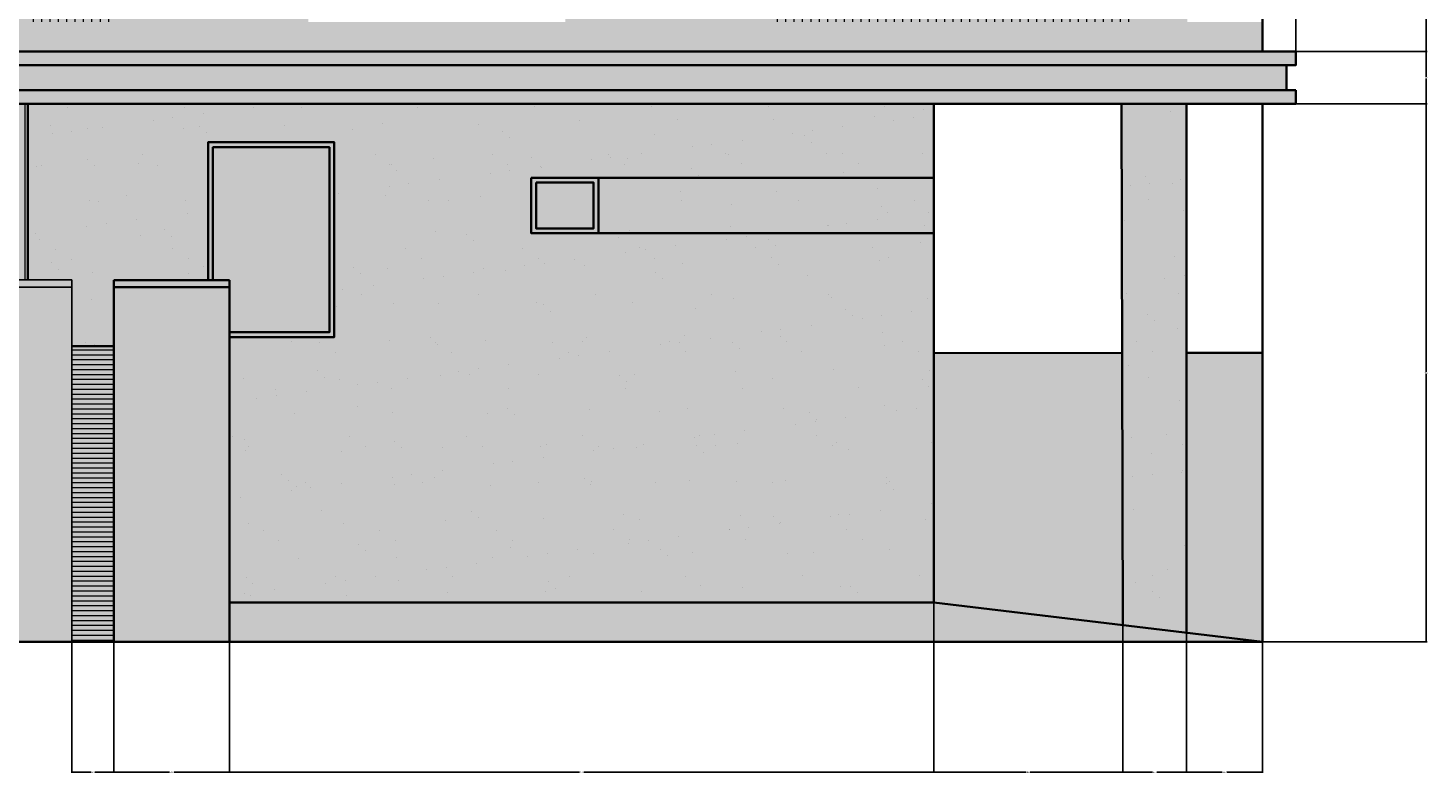
# Model space of a CAD drawing. Units: feet. Extents: x 2651 to 4047, y 949 to 1287.
# Tile 2 of 5: x 2945 to 3230, y 949 to 1100. Entities that reach past the tile are written whole.
import ezdxf

# ---------------------------------------------------------------- set-up
doc = ezdxf.new("R2010")
doc.units = ezdxf.units.FT
for name, color, linetype, lineweight in [('A-ANNO-DIMS', 2, 'Continuous', 18), ('A-ELEV', 7, 'Continuous', 35), ('A-ELEV-FNCE', 7, 'Continuous', 25), ('A-ELEV-PATT', 8, 'Continuous', 13)]:
    doc.layers.add(name, color=color, linetype=linetype, lineweight=lineweight)
doc.styles.get("Standard").update_dxf_attribs({"font": 'arial.ttf'})
doc.dimstyles.get("Standard").update_dxf_attribs({"dimtxt": 0.18, "dimasz": 0.18, "dimexe": 0.18, "dimexo": 0.0625, "dimgap": 0.09, "dimtad": 0, "dimtih": 1, "dimtoh": 1, "dimdec": 1, "dimzin": 0, "dimdsep": 46, "dimlunit": 3, "dimtxsty": 'Standard', "dimcen": 0.09, "dimadec": 0, "dimazin": 0, "dimtfac": 1, "dimtdec": 1, "dimtofl": 0, "dimtmove": 0, "dimatfit": 3, "dimfxl": 1, "dimtolj": 1, "dimtzin": 0, "dimarcsym": 0})

# ---------------------------------------------------------------- blocks, each defined once
blk = doc.blocks.new('BOUNDARY-PIER-HATCHED')
for p, q in [((0, 72.1), (0, 73.54)), ((0, 72.1), (0, 73.54)), ((12.86, 0), (12.86, 73.54)), ((12.86, 0), (12.86, 73.54))]:
    blk.add_line(p, q)
for points in [[(0, 73.54), (12.86, 73.54)], [(0, 73.54), (12.86, 73.54)], [(12.86, 72.1), (0, 72.1)], [(12.86, 0), (0, 0), (0, 72.1), (12.86, 72.1)], [(12.86, 0), (0, 0), (0, 72.1), (12.86, 72.1)], [(12.86, 72.1), (0, 72.1)]]:
    blk.add_lwpolyline(points)
blk = doc.blocks.new('*D7')
at = {"layer": 'A-ANNO-DIMS', "color": 0, "lineweight": -2, "transparency": 16777216}
for p, q in [((2677.56, 975.71), (2677.56, 1287.01)), ((2677.74, 1286.83), (2939.77, 1286.83)), ((3202.59, 1286.83), (2940.56, 1286.83)), ((3202.77, 1095.71), (3202.77, 1287.01))]:
    blk.add_line(p, q, dxfattribs=at)
at = {"layer": 'A-ANNO-DIMS', "color": 0, "transparency": 16777216}
for points in [[(2677.74, 1286.86), (2677.74, 1286.8), (2677.56, 1286.83)], [(3202.59, 1286.86), (3202.59, 1286.8), (3202.77, 1286.83)]]:
    blk.add_solid(points, dxfattribs=at)
at = {"layer": 'Defpoints', "color": 0, "transparency": 16777216}
for p in [(3202.77, 1286.83), (3202.77, 1095.65), (2677.56, 975.65)]:
    blk.add_point(p, dxfattribs=at)
at = {"layer": 'A-ANNO-DIMS', "color": 0, "transparency": 16777216, "insert": (2940.17, 1286.83), "char_height": 0.18, "attachment_point": 5}
blk.add_mtext('\\A1;525.2', dxfattribs=at)
blk = doc.blocks.new('*D8')
at = {"layer": 'A-ANNO-DIMS', "color": 0, "lineweight": -2, "transparency": 16777216}
for p, q in [((3098.48, 1260.33), (2650.88, 1260.33)), ((2651.06, 1260.15), (2651.06, 1118.17)), ((2651.06, 975.83), (2651.06, 1117.81)), ((2677.49, 975.65), (2650.88, 975.65))]:
    blk.add_line(p, q, dxfattribs=at)
at = {"layer": 'A-ANNO-DIMS', "color": 0, "transparency": 16777216}
for points in [[(2651.03, 1260.15), (2651.09, 1260.15), (2651.06, 1260.33)], [(2651.03, 975.83), (2651.09, 975.83), (2651.06, 975.65)]]:
    blk.add_solid(points, dxfattribs=at)
at = {"layer": 'Defpoints', "color": 0, "transparency": 16777216}
for p in [(2651.06, 1260.33), (3098.55, 1260.33), (2677.56, 975.65)]:
    blk.add_point(p, dxfattribs=at)
at = {"layer": 'A-ANNO-DIMS', "color": 0, "transparency": 16777216, "insert": (2651.06, 1117.99), "char_height": 0.18, "attachment_point": 5}
blk.add_mtext('\\A1;284.7', dxfattribs=at)
blk = doc.blocks.new('*D14')
at = {"layer": 'A-ANNO-DIMS', "color": 0, "lineweight": -2, "transparency": 16777216}
for p, q in [((2953.89, 975.59), (2953.89, 948.97)), ((2962.47, 975.59), (2962.47, 948.97)), ((2954.07, 949.15), (2957.78, 949.15)), ((2962.29, 949.15), (2958.57, 949.15))]:
    blk.add_line(p, q, dxfattribs=at)
at = {"layer": 'A-ANNO-DIMS', "color": 0, "transparency": 16777216}
for points in [[(2954.07, 949.18), (2954.07, 949.12), (2953.89, 949.15)], [(2962.29, 949.18), (2962.29, 949.12), (2962.47, 949.15)]]:
    blk.add_solid(points, dxfattribs=at)
at = {"layer": 'Defpoints', "color": 0, "transparency": 16777216}
for p in [(2953.89, 975.65), (2962.47, 975.65), (2962.47, 949.15)]:
    blk.add_point(p, dxfattribs=at)
at = {"layer": 'A-ANNO-DIMS', "color": 0, "transparency": 16777216, "insert": (2958.18, 949.15), "char_height": 0.18, "attachment_point": 5}
blk.add_mtext('\\A1;8.576', dxfattribs=at)
blk = doc.blocks.new('*D15')
at = {"layer": 'A-ANNO-DIMS', "color": 0, "lineweight": -2, "transparency": 16777216}
for p, q in [((2962.47, 975.59), (2962.47, 948.97)), ((2985.99, 975.59), (2985.99, 948.97)), ((2962.65, 949.15), (2973.76, 949.15)), ((2985.81, 949.15), (2974.69, 949.15))]:
    blk.add_line(p, q, dxfattribs=at)
at = {"layer": 'A-ANNO-DIMS', "color": 0, "transparency": 16777216}
for points in [[(2962.65, 949.18), (2962.65, 949.12), (2962.47, 949.15)], [(2985.81, 949.18), (2985.81, 949.12), (2985.99, 949.15)]]:
    blk.add_solid(points, dxfattribs=at)
at = {"layer": 'Defpoints', "color": 0, "transparency": 16777216}
for p in [(2962.47, 975.65), (2985.99, 975.65), (2985.99, 949.15)]:
    blk.add_point(p, dxfattribs=at)
at = {"layer": 'A-ANNO-DIMS', "color": 0, "transparency": 16777216, "insert": (2974.23, 949.15), "char_height": 0.18, "attachment_point": 5}
blk.add_mtext('\\A1;23.525', dxfattribs=at)
blk = doc.blocks.new('*D16')
at = {"layer": 'A-ANNO-DIMS', "color": 0, "lineweight": -2, "transparency": 16777216}
for p, q in [((2985.99, 983.55), (2985.99, 948.97)), ((3129.15, 983.55), (3129.15, 948.97)), ((2986.17, 949.15), (3057.12, 949.15)), ((3128.97, 949.15), (3058.03, 949.15))]:
    blk.add_line(p, q, dxfattribs=at)
at = {"layer": 'A-ANNO-DIMS', "color": 0, "transparency": 16777216}
for points in [[(2986.17, 949.18), (2986.17, 949.12), (2985.99, 949.15)], [(3128.97, 949.18), (3128.97, 949.12), (3129.15, 949.15)]]:
    blk.add_solid(points, dxfattribs=at)
at = {"layer": 'Defpoints', "color": 0, "transparency": 16777216}
for p in [(2985.99, 983.61), (3129.15, 983.61), (3129.15, 949.15)]:
    blk.add_point(p, dxfattribs=at)
at = {"layer": 'A-ANNO-DIMS', "color": 0, "transparency": 16777216, "insert": (3057.57, 949.15), "char_height": 0.18, "attachment_point": 5}
blk.add_mtext('\\A1;143.16', dxfattribs=at)
blk = doc.blocks.new('*D17')
at = {"layer": 'A-ANNO-DIMS', "color": 0, "lineweight": -2, "transparency": 16777216}
for p, q in [((3129.15, 983.55), (3129.15, 948.97)), ((3167.58, 978.97), (3167.58, 948.97)), ((3129.33, 949.15), (3147.97, 949.15)), ((3167.4, 949.15), (3148.76, 949.15))]:
    blk.add_line(p, q, dxfattribs=at)
at = {"layer": 'A-ANNO-DIMS', "color": 0, "transparency": 16777216}
for points in [[(3129.33, 949.18), (3129.33, 949.12), (3129.15, 949.15)], [(3167.4, 949.18), (3167.4, 949.12), (3167.58, 949.15)]]:
    blk.add_solid(points, dxfattribs=at)
at = {"layer": 'Defpoints', "color": 0, "transparency": 16777216}
for p in [(3129.15, 983.61), (3167.58, 979.04), (3167.58, 949.15)]:
    blk.add_point(p, dxfattribs=at)
at = {"layer": 'A-ANNO-DIMS', "color": 0, "transparency": 16777216, "insert": (3148.36, 949.15), "char_height": 0.18, "attachment_point": 5}
blk.add_mtext('\\A1;38.42', dxfattribs=at)
blk = doc.blocks.new('*D18')
at = {"layer": 'A-ANNO-DIMS', "color": 0, "lineweight": -2, "transparency": 16777216}
for p, q in [((3167.58, 978.97), (3167.58, 948.97)), ((3180.54, 977.43), (3180.54, 948.97)), ((3167.76, 949.15), (3173.6, 949.15)), ((3180.36, 949.15), (3174.51, 949.15))]:
    blk.add_line(p, q, dxfattribs=at)
at = {"layer": 'A-ANNO-DIMS', "color": 0, "transparency": 16777216}
for points in [[(3167.76, 949.18), (3167.76, 949.12), (3167.58, 949.15)], [(3180.36, 949.18), (3180.36, 949.12), (3180.54, 949.15)]]:
    blk.add_solid(points, dxfattribs=at)
at = {"layer": 'Defpoints', "color": 0, "transparency": 16777216}
for p in [(3167.58, 979.04), (3180.54, 977.49), (3180.54, 949.15)]:
    blk.add_point(p, dxfattribs=at)
at = {"layer": 'A-ANNO-DIMS', "color": 0, "transparency": 16777216, "insert": (3174.06, 949.15), "char_height": 0.18, "attachment_point": 5}
blk.add_mtext('\\A1;12.966', dxfattribs=at)
blk = doc.blocks.new('*D19')
at = {"layer": 'A-ANNO-DIMS', "color": 0, "lineweight": -2, "transparency": 16777216}
for p, q in [((3180.54, 977.43), (3180.54, 948.97)), ((3196.01, 975.59), (3196.01, 948.97)), ((3180.72, 949.15), (3187.82, 949.15)), ((3195.83, 949.15), (3188.73, 949.15))]:
    blk.add_line(p, q, dxfattribs=at)
at = {"layer": 'A-ANNO-DIMS', "color": 0, "transparency": 16777216}
for points in [[(3180.72, 949.18), (3180.72, 949.12), (3180.54, 949.15)], [(3195.83, 949.18), (3195.83, 949.12), (3196.01, 949.15)]]:
    blk.add_solid(points, dxfattribs=at)
at = {"layer": 'Defpoints', "color": 0, "transparency": 16777216}
for p in [(3180.54, 977.49), (3196.01, 975.65), (3196.01, 949.15)]:
    blk.add_point(p, dxfattribs=at)
at = {"layer": 'A-ANNO-DIMS', "color": 0, "transparency": 16777216, "insert": (3188.28, 949.15), "char_height": 0.18, "attachment_point": 5}
blk.add_mtext('\\A1;15.467', dxfattribs=at)
blk = doc.blocks.new('*D20')
at = {"layer": 'A-ANNO-DIMS', "color": 0, "lineweight": -2, "transparency": 16777216}
for p, q in [((3202.84, 1084.98), (3229.45, 1084.98)), ((3229.27, 1084.8), (3229.27, 1030.5)), ((3229.27, 975.83), (3229.27, 1030.13)), ((3196.07, 975.65), (3229.45, 975.65))]:
    blk.add_line(p, q, dxfattribs=at)
at = {"layer": 'A-ANNO-DIMS', "color": 0, "transparency": 16777216}
for points in [[(3229.24, 1084.8), (3229.3, 1084.8), (3229.27, 1084.98)], [(3229.24, 975.83), (3229.3, 975.83), (3229.27, 975.65)]]:
    blk.add_solid(points, dxfattribs=at)
at = {"layer": 'Defpoints', "color": 0, "transparency": 16777216}
for p in [(3202.77, 1084.98), (3229.27, 1084.98), (3196.01, 975.65)]:
    blk.add_point(p, dxfattribs=at)
at = {"layer": 'A-ANNO-DIMS', "color": 0, "transparency": 16777216, "insert": (3229.27, 1030.31), "char_height": 0.18, "attachment_point": 5}
blk.add_mtext('\\A1;109.33', dxfattribs=at)
blk = doc.blocks.new('*D21')
at = {"layer": 'A-ANNO-DIMS', "color": 0, "lineweight": -2, "transparency": 16777216}
for p, q in [((3202.84, 1095.65), (3229.45, 1095.65)), ((3229.27, 1095.47), (3229.27, 1090.5)), ((3229.27, 1085.16), (3229.27, 1090.13)), ((3202.84, 1084.98), (3229.45, 1084.98))]:
    blk.add_line(p, q, dxfattribs=at)
at = {"layer": 'A-ANNO-DIMS', "color": 0, "transparency": 16777216}
for points in [[(3229.24, 1095.47), (3229.3, 1095.47), (3229.27, 1095.65)], [(3229.24, 1085.16), (3229.3, 1085.16), (3229.27, 1084.98)]]:
    blk.add_solid(points, dxfattribs=at)
at = {"layer": 'Defpoints', "color": 0, "transparency": 16777216}
for p in [(3202.77, 1095.65), (3229.27, 1095.65), (3202.77, 1084.98)]:
    blk.add_point(p, dxfattribs=at)
at = {"layer": 'A-ANNO-DIMS', "color": 0, "transparency": 16777216, "insert": (3229.27, 1090.31), "char_height": 0.18, "attachment_point": 5}
blk.add_mtext('\\A1;10.673', dxfattribs=at)
blk = doc.blocks.new('*D22')
at = {"layer": 'A-ANNO-DIMS', "color": 0, "lineweight": -2, "transparency": 16777216}
for p, q in [((3196.07, 1127.71), (3229.45, 1127.71)), ((3229.27, 1127.53), (3229.27, 1111.86)), ((3229.27, 1095.83), (3229.27, 1111.5)), ((3196.07, 1095.65), (3229.45, 1095.65))]:
    blk.add_line(p, q, dxfattribs=at)
at = {"layer": 'A-ANNO-DIMS', "color": 0, "transparency": 16777216}
for points in [[(3229.24, 1127.53), (3229.3, 1127.53), (3229.27, 1127.71)], [(3229.24, 1095.83), (3229.3, 1095.83), (3229.27, 1095.65)]]:
    blk.add_solid(points, dxfattribs=at)
at = {"layer": 'Defpoints', "color": 0, "transparency": 16777216}
for p in [(3196.01, 1127.71), (3229.27, 1127.71), (3196.01, 1095.65)]:
    blk.add_point(p, dxfattribs=at)
at = {"layer": 'A-ANNO-DIMS', "color": 0, "transparency": 16777216, "insert": (3229.27, 1111.68), "char_height": 0.18, "attachment_point": 5}
blk.add_mtext('\\A1;32.06', dxfattribs=at)

msp = doc.modelspace()

# ---------------------------------------------------------------- hatches: boundary and pattern name
at = {"layer": 'A-ELEV-PATT'}
h = msp.add_hatch(color=256, dxfattribs=at)
h.dxf.hatch_style = 1
h.paths.add_polyline_path([(2944.9934, 1227.65), (2896.1919, 1227.65), (2707.3507, 1227.65), (2707.3507, 1221.65), (2938.9934, 1221.65), (2938.9934, 1127.711), (2944.9934, 1127.711), (2944.9934, 1221.65)])
h.paths.add_polyline_path([(2944.9934, 1127.711), (2938.9934, 1127.711), (2938.9934, 1101.65), (2938.9934, 1095.65), (3196.0086, 1095.65), (3196.0086, 1101.65), (3180.6945, 1101.65), (3180.6945, 1127.711), (3169.7582, 1127.711), (3169.7582, 1101.65), (3097.3565, 1101.65), (3002.0224, 1101.65), (2944.9934, 1101.65)])
h.paths.add_polyline_path([(3180.6945, 1242.6921), (3169.7582, 1242.6921), (3169.7582, 1221.65), (3169.7582, 1127.711), (3180.6945, 1127.711)])
h = msp.add_hatch(color=256, dxfattribs=at)
h.set_gradient(color1=(199, 200, 202), color2=(199, 200, 202), tint=1, name='HEMISPHERICAL')
h.paths.add_polyline_path([(2763.5286, 1190.8721), (2719.1033, 1190.8721), (2719.1033, 1152.9072), (2763.5286, 1152.9072)])
h.paths.add_polyline_path([(2838.0977, 1190.8721), (2763.5286, 1190.8721), (2763.5286, 1152.9072), (2838.0977, 1152.9072)])
h.paths.add_polyline_path([(2887.0237, 1190.8721), (2838.0977, 1190.8721), (2838.0977, 1152.9072), (2887.0237, 1152.9072)])
h.paths.add_polyline_path([(2877.0224, 1127.711), (2887.0237, 1127.711), (2887.0237, 1152.9072), (2838.0977, 1152.9072), (2838.0977, 1099.175), (2839.8136, 1099.175), (2839.8136, 1098.3392), (2838.0977, 1098.3392), (2838.0977, 1093.6891), (2839.8136, 1093.6891), (2839.8136, 1092.8533), (2872.1973, 1092.8533), (2872.1973, 1095.65), (2877.0224, 1095.65)])
h.paths.add_polyline_path([(2887.0237, 1127.711), (2877.0224, 1127.711), (2877.0224, 1095.65), (2887.0237, 1095.65)], flags=17)
h.paths.add_polyline_path([(2887.0237, 1084.9772), (2872.1973, 1084.9772), (2872.1973, 1087.7738), (2873.8204, 1087.7738), (2873.8204, 1092.8533), (2872.1973, 1092.8533), (2838.0977, 1092.8533), (2838.0977, 1049.1862), (2887.0237, 1049.1862)])
h.paths.add_polyline_path([(2763.5286, 1152.9072), (2719.1033, 1152.9072), (2719.1033, 1092.8533), (2761.8127, 1092.8533), (2761.8127, 1093.6891), (2763.5286, 1093.6891), (2763.5286, 1098.3392), (2761.8127, 1098.3392), (2761.8127, 1099.175), (2763.5286, 1099.175)])
h.paths.add_polyline_path([(2763.5286, 1092.8533), (2719.1033, 1092.8533), (2719.1033, 1049.1862), (2763.5286, 1049.1862), (2763.5286, 1072.7574)])
h.paths.add_polyline_path([(2838.0977, 1152.9072), (2763.5286, 1152.9072), (2763.5286, 1148.4143), (2838.0977, 1148.4143)])
h.paths.add_polyline_path([(2838.0977, 1092.8533), (2763.5286, 1092.8533), (2763.5286, 1072.7574), (2838.0977, 1072.7574)])
h.paths.add_polyline_path([(2883.0637, 1047.7503), (2677.5561, 1047.7503), (2677.5561, 1035.7503), (2871.0637, 1035.7503), (2871.0637, 975.65), (2883.0637, 975.65)])
h.paths.add_polyline_path([(2911.0266, 1047.7503), (2898.171, 1047.7503), (2898.171, 975.65), (2911.0266, 975.65)])
h.paths.add_polyline_path([(2932.4585, 1047.7503), (2919.6029, 1047.7503), (2919.6029, 975.65), (2932.4585, 975.65)])
h.paths.add_polyline_path([(2953.8904, 1047.7503), (2941.0349, 1047.7503), (2941.0349, 975.65), (2953.8904, 975.65)])
h.paths.add_polyline_path([(2985.9915, 1047.7503), (2962.4668, 1047.7503), (2962.4668, 975.65), (2975.3223, 975.65), (2985.9915, 975.65)])
h.paths.add_polyline_path([(3097.3565, 1221.65), (3097.3565, 1238.6943), (3054.2372, 1238.6943), (3054.2372, 1163.1131), (3097.3565, 1163.1131)])
h.paths.add_polyline_path([(3002.0224, 1238.6943), (2962.7341, 1238.6943), (2962.7341, 1163.1131), (3002.0224, 1163.1131)])
h.paths.add_polyline_path([(3054.2372, 1238.6943), (3002.0224, 1238.6943), (3002.0224, 1163.1131), (3054.2372, 1163.1131)])
h.paths.add_polyline_path([(3002.0224, 1163.1131), (2962.7341, 1163.1131), (2962.7341, 1127.711), (3002.0224, 1127.711)])
h.paths.add_polyline_path([(3002.0224, 1127.711), (2962.7341, 1127.711), (2962.7341, 1101.65), (3002.0224, 1101.65)])
h.paths.add_polyline_path([(3097.3565, 1163.1131), (3054.2372, 1163.1131), (3054.2372, 1127.711), (3097.3565, 1127.711)])
h.paths.add_polyline_path([(3097.3565, 1127.711), (3054.2372, 1127.711), (3054.2372, 1101.65), (3097.3565, 1101.65)])
h = msp.add_hatch(color=256, dxfattribs=at)
h.set_gradient(color1=(168, 95, 18), color2=(168, 95, 18), tint=1, name='CURVED')
h.paths.add_polyline_path([(2938.9934, 1207.954), (2732.0644, 1207.954), (2732.0644, 1190.8721), (2887.0237, 1190.8721), (2887.0237, 1127.711), (2938.9934, 1127.711)])
h.paths.add_polyline_path([(2938.9934, 1221.65), (2707.3507, 1221.65), (2732.0644, 1207.954), (2938.9934, 1207.954)])
h.paths.add_polyline_path([(3169.7582, 1221.65), (3097.3565, 1221.65), (3097.3565, 1127.711), (3169.7582, 1127.711)])
h.paths.add_polyline_path([(2962.7341, 1221.65), (2944.9934, 1221.65), (2944.9934, 1127.711), (2962.7341, 1127.711)])
h.paths.add_polyline_path([(3169.7582, 1227.65), (3097.3565, 1227.65), (3097.3565, 1221.65), (3169.7582, 1221.65)])
h.paths.add_polyline_path([(3169.7582, 1127.711), (3097.3565, 1127.711), (3097.3565, 1101.65), (3169.7582, 1101.65)])
h.paths.add_polyline_path([(2962.7341, 1127.711), (2944.9934, 1127.711), (2944.9934, 1101.65), (2962.7341, 1101.65)])
h.paths.add_polyline_path([(2938.9934, 1127.711), (2887.0237, 1127.711), (2887.0237, 1095.65), (2938.9934, 1095.65), (2938.9934, 1101.65)])
h.paths.add_polyline_path([(2944.9934, 1084.9772), (2887.0237, 1084.9772), (2887.0237, 1049.1862), (2883.0637, 1049.1862), (2883.0637, 1047.7503), (2883.0637, 1035.7503), (2898.171, 1035.7503), (2898.171, 1047.7503), (2898.171, 1049.1862), (2911.0266, 1049.1862), (2911.0266, 1035.7503), (2919.6029, 1035.7503), (2919.6029, 1047.7503), (2919.6029, 1049.1862), (2932.4585, 1049.1862), (2932.4585, 1035.7503), (2941.0349, 1035.7503), (2941.0349, 1047.7503), (2941.0349, 1049.1862), (2944.9934, 1049.1862)])
h = msp.add_hatch(dxfattribs=at)
h.set_pattern_fill('_USER', color=256, scale=1.7, angle=90, style=0, pattern_type=0)
h.set_pattern_definition([(90, (0, 0), (-1.7, 1e-16), [])])
h.paths.add_polyline_path([(2938.9934, 1207.954), (2732.0644, 1207.954), (2732.0644, 1190.8721), (2887.0237, 1190.8721), (2887.0237, 1127.711), (2938.9934, 1127.711)])
h.paths.add_polyline_path([(2938.9934, 1221.65), (2707.3507, 1221.65), (2732.0644, 1207.954), (2938.9934, 1207.954)])
h.paths.add_polyline_path([(2938.9934, 1127.711), (2887.0237, 1127.711), (2887.0237, 1095.65), (2938.9934, 1095.65), (2938.9934, 1101.65)])
h.paths.add_polyline_path([(2962.7341, 1221.65), (2944.9934, 1221.65), (2944.9934, 1127.711), (2962.7341, 1127.711)])
h.paths.add_polyline_path([(2962.7341, 1127.711), (2944.9934, 1127.711), (2944.9934, 1101.65), (2962.7341, 1101.65)])
h.paths.add_polyline_path([(3169.7582, 1221.65), (3097.3565, 1221.65), (3097.3565, 1127.711), (3169.7582, 1127.711)])
h.paths.add_polyline_path([(3169.7582, 1227.65), (3097.3565, 1227.65), (3097.3565, 1221.65), (3169.7582, 1221.65)])
h.paths.add_polyline_path([(3169.7582, 1127.711), (3097.3565, 1127.711), (3097.3565, 1101.65), (3169.7582, 1101.65)])
h.paths.add_polyline_path([(2944.9934, 1084.9772), (2887.0237, 1084.9772), (2887.0237, 1049.1862), (2883.0637, 1049.1862), (2883.0637, 1047.7503), (2883.0637, 1035.7503), (2898.171, 1035.7503), (2898.171, 1047.7503), (2898.171, 1049.1862), (2911.0266, 1049.1862), (2911.0266, 1035.7503), (2919.6029, 1035.7503), (2919.6029, 1047.7503), (2919.6029, 1049.1862), (2932.4585, 1049.1862), (2932.4585, 1035.7503), (2941.0349, 1035.7503), (2941.0349, 1047.7503), (2941.0349, 1049.1862), (2944.9934, 1049.1862)])
h = msp.add_hatch(dxfattribs=at)
h.set_pattern_fill('AR-SAND', color=256, scale=0.09, style=0)
h.set_pattern_definition([(37.5, (-817.72, 3e-12), (-0.1440028, 4.404719), [0, -3.47472, 0, -3.8862, 0, -3.71475]), (7.5, (-817.72, 3e-12), (4.0457095, 6.451426), [0, -1.87452, 0, -3.13182, 0, -1.20015]), (327.5, (-820.5318, 3e-12), (7.1189313, 0.0129347), [0, -1.143, 0, -4.1148, 0, -5.3721]), (317.5, (-820.532, 3e-12), (6.872008, 2.006364), [0, -0.5715, 0, -2.69748, 0, -3.0861])])
h.paths.add_polyline_path([(2763.5286, 1190.8721), (2719.1033, 1190.8721), (2719.1033, 1152.9072), (2763.5286, 1152.9072)])
h.paths.add_polyline_path([(2838.0977, 1190.8721), (2763.5286, 1190.8721), (2763.5286, 1152.9072), (2838.0977, 1152.9072)])
h.paths.add_polyline_path([(2887.0237, 1190.8721), (2838.0977, 1190.8721), (2838.0977, 1152.9072), (2887.0237, 1152.9072)])
h.paths.add_polyline_path([(2838.0977, 1152.9072), (2763.5286, 1152.9072), (2763.5286, 1148.4143), (2838.0977, 1148.4143)])
h.paths.add_polyline_path([(2887.0237, 1152.9072), (2838.0977, 1152.9072), (2838.0977, 1099.175), (2839.8136, 1099.175), (2839.8136, 1098.3392), (2838.0977, 1098.3392), (2838.0977, 1093.6891), (2839.8136, 1093.6891), (2839.8136, 1092.8533), (2872.1973, 1092.8533), (2872.1973, 1095.65), (2877.0224, 1095.65), (2877.0224, 1127.711), (2887.0237, 1127.711)])
h.paths.add_polyline_path([(2887.0237, 1127.711), (2877.0224, 1127.711), (2877.0224, 1095.65), (2887.0237, 1095.65)], flags=17)
h.paths.add_polyline_path([(2763.5286, 1152.9072), (2719.1033, 1152.9072), (2719.1033, 1092.8533), (2761.8127, 1092.8533), (2761.8127, 1093.6891), (2763.5286, 1093.6891), (2763.5286, 1098.3392), (2761.8127, 1098.3392), (2761.8127, 1099.175), (2763.5286, 1099.175)])
h.paths.add_polyline_path([(2763.5286, 1092.8533), (2761.8127, 1092.8533), (2719.1033, 1092.8533), (2719.1033, 1049.1862), (2763.5286, 1049.1862)])
h.paths.add_polyline_path([(2887.0237, 1084.9772), (2872.1973, 1084.9772), (2872.1973, 1087.7738), (2873.8204, 1087.7738), (2873.8204, 1092.8533), (2872.1973, 1092.8533), (2838.0977, 1092.8533), (2838.0977, 1049.1862), (2887.0237, 1049.1862)])
h.paths.add_polyline_path([(2838.0977, 1092.8533), (2763.5286, 1092.8533), (2763.5286, 1072.7574), (2838.0977, 1072.7574)])
h.paths.add_polyline_path([(2911.0266, 1047.7503), (2898.171, 1047.7503), (2898.171, 975.65), (2911.0266, 975.65)])
h.paths.add_polyline_path([(2932.4585, 1047.7503), (2919.6029, 1047.7503), (2919.6029, 975.65), (2932.4585, 975.65)])
h.paths.add_polyline_path([(2953.8904, 1047.7503), (2941.0349, 1047.7503), (2941.0349, 975.65), (2953.8904, 975.65)])
h.paths.add_polyline_path([(2985.9915, 1047.7503), (2962.4668, 1047.7503), (2962.4668, 975.65), (2975.3223, 975.65), (2985.9915, 975.65)])
h.paths.add_polyline_path([(2883.0637, 1047.7503), (2677.5561, 1047.7503), (2677.5561, 1035.7503), (2871.0637, 1035.7503), (2871.0637, 975.65), (2883.0637, 975.65)])
h = msp.add_hatch(color=256, dxfattribs=at)
h.paths.add_polyline_path([(2838.0977, 1148.4143), (2763.5286, 1148.4143), (2763.5286, 1099.175), (2838.0977, 1099.175)])
h.paths.add_polyline_path([(2836.0977, 1146.4143), (2836.0977, 1101.175), (2765.5286, 1101.175), (2765.5286, 1146.4143)], flags=16)
h.paths.add_polyline_path([(2819.7437, 1135.9058), (2819.7437, 1113.3773), (2782.111, 1113.3773), (2782.111, 1135.9058)], flags=0)
h.paths.add_polyline_path([(2819.1363, 1135.3515), (2819.1363, 1113.9316), (2782.7185, 1113.9316), (2782.7185, 1135.3515)], flags=0)
h.paths.add_polyline_path([(2782.7185, 1146.4143), (2782.111, 1146.4143), (2782.111, 1135.9058), (2782.7185, 1135.9058)], flags=0)
h.paths.add_polyline_path([(2782.111, 1135.9058), (2765.5286, 1135.9058), (2765.5286, 1135.3515), (2782.111, 1135.3515)], flags=0)
h.paths.add_polyline_path([(2836.0977, 1135.9058), (2819.7437, 1135.9058), (2819.7437, 1135.3515), (2836.0977, 1135.3515)], flags=0)
h.paths.add_polyline_path([(2819.7437, 1146.4143), (2819.1363, 1146.4143), (2819.1363, 1135.9058), (2819.7437, 1135.9058)], flags=0)
h.paths.add_polyline_path([(2836.0977, 1113.9316), (2819.7437, 1113.9316), (2819.7437, 1113.3773), (2836.0977, 1113.3773)], flags=0)
h.paths.add_polyline_path([(2819.7437, 1113.3773), (2819.1363, 1113.3773), (2819.1363, 1101.175), (2819.7437, 1101.175)], flags=0)
h.paths.add_polyline_path([(2782.111, 1113.9316), (2765.5286, 1113.9316), (2765.5286, 1113.3773), (2782.111, 1113.3773)], flags=0)
h.paths.add_polyline_path([(2782.7185, 1113.3773), (2782.111, 1113.3773), (2782.111, 1101.175), (2782.7185, 1101.175)], flags=0)
h.paths.add_polyline_path([(2781.7185, 1061.2489), (2781.111, 1061.2489), (2781.111, 1060.6946), (2781.7185, 1060.6946)])
h.paths.add_polyline_path([(2781.7185, 1072.7574), (2781.111, 1072.7574), (2781.111, 1061.2489), (2781.7185, 1061.2489)])
h.paths.add_polyline_path([(2838.0977, 1061.2489), (2781.7185, 1061.2489), (2781.7185, 1060.6946), (2838.0977, 1060.6946)])
h.paths.add_polyline_path([(2781.111, 1061.2489), (2763.5286, 1061.2489), (2763.5286, 1060.6946), (2781.111, 1060.6946)])
h.paths.add_polyline_path([(2781.7185, 1060.6946), (2781.111, 1060.6946), (2781.111, 1049.1862), (2781.7185, 1049.1862)])
h.paths.add_polyline_path([(2781.111, 1072.7574), (2763.5286, 1072.7574), (2763.5286, 1061.2489), (2764.5286, 1061.2489), (2764.5286, 1071.7574), (2781.111, 1071.7574)])
h.paths.add_polyline_path([(2838.0977, 1072.7574), (2781.7185, 1072.7574), (2781.7185, 1071.7574), (2837.0977, 1071.7574), (2837.0977, 1061.2489), (2838.0977, 1061.2489)])
h.paths.add_polyline_path([(2838.0977, 1060.6946), (2837.0977, 1060.6946), (2837.0977, 1050.1862), (2781.7185, 1050.1862), (2781.7185, 1049.1862), (2838.0977, 1049.1862)])
h.paths.add_polyline_path([(2764.5286, 1060.6946), (2763.5286, 1060.6946), (2763.5286, 1049.1862), (2781.111, 1049.1862), (2781.111, 1050.1862), (2764.5286, 1050.1862)])
h.paths.add_polyline_path([(2818.7437, 1071.7574), (2818.1363, 1071.7574), (2818.1363, 1061.2489), (2818.7437, 1061.2489)], flags=17)
h.paths.add_polyline_path([(2818.7437, 1060.6946), (2818.1363, 1060.6946), (2818.1363, 1050.1862), (2818.7437, 1050.1862)], flags=17)
h.paths.add_polyline_path([(2883.0637, 1049.1862), (2719.1033, 1049.1862), (2677.5561, 1049.1862), (2677.5561, 1047.7503), (2883.0637, 1047.7503)])
h.paths.add_polyline_path([(2911.0266, 1049.1862), (2898.171, 1049.1862), (2898.171, 1047.7503), (2911.0266, 1047.7503)])
h.paths.add_polyline_path([(2932.4585, 1049.1862), (2919.6029, 1049.1862), (2919.6029, 1047.7503), (2932.4585, 1047.7503)])
h.paths.add_polyline_path([(2953.8904, 1049.1862), (2941.0349, 1049.1862), (2941.0349, 1047.7503), (2953.8904, 1047.7503)])
h.paths.add_polyline_path([(2985.9915, 1049.1862), (2962.4668, 1049.1862), (2962.4668, 1047.7503), (2985.9915, 1047.7503)])
h.paths.add_polyline_path([(3007.2777, 1077.1763), (2981.6074, 1077.1763), (2981.6074, 1049.1862), (2982.6074, 1049.1862), (2982.6074, 1076.1763), (3006.2777, 1076.1763), (3006.2777, 1038.5677), (2985.9915, 1038.5677), (2985.9915, 1037.5677), (3007.2777, 1037.5677)])
h.paths.add_polyline_path([(3060.9744, 1069.9768), (3047.3083, 1069.9768), (3047.3083, 1058.6821), (3060.9744, 1058.6821)])
h.paths.add_polyline_path([(3059.9744, 1068.9768), (3059.9744, 1059.6821), (3048.3083, 1059.6821), (3048.3083, 1068.9768)], flags=16)
h = msp.add_hatch(color=256, dxfattribs=at)
h.set_gradient(color1=(194, 211, 228), color2=(194, 211, 228), name='HEMISPHERICAL')
h.paths.add_polyline_path([(2819.1363, 1135.3515), (2782.7185, 1135.3515), (2782.7185, 1113.9316), (2819.1363, 1113.9316)])
h.paths.add_polyline_path([(2782.111, 1146.4143), (2765.5286, 1146.4143), (2765.5286, 1135.9058), (2782.111, 1135.9058)])
h.paths.add_polyline_path([(2819.1363, 1146.4143), (2782.7185, 1146.4143), (2782.7185, 1135.9058), (2819.1363, 1135.9058)])
h.paths.add_polyline_path([(2782.111, 1135.3515), (2765.5286, 1135.3515), (2765.5286, 1113.9316), (2782.111, 1113.9316)])
h.paths.add_polyline_path([(2836.0977, 1146.4143), (2819.7437, 1146.4143), (2819.7437, 1135.9058), (2836.0977, 1135.9058)])
h.paths.add_polyline_path([(2836.0977, 1135.3515), (2819.7437, 1135.3515), (2819.7437, 1113.9316), (2836.0977, 1113.9316)])
h.paths.add_polyline_path([(2836.0977, 1113.3773), (2819.7437, 1113.3773), (2819.7437, 1101.175), (2836.0977, 1101.175)])
h.paths.add_polyline_path([(2819.1363, 1113.3773), (2782.7185, 1113.3773), (2782.7185, 1101.175), (2819.1363, 1101.175)])
h.paths.add_polyline_path([(2782.111, 1113.3773), (2765.5286, 1113.3773), (2765.5286, 1101.175), (2782.111, 1101.175)])
h.paths.add_polyline_path([(2781.111, 1060.6946), (2764.5286, 1060.6946), (2764.5286, 1050.1862), (2781.111, 1050.1862)])
h.paths.add_polyline_path([(2818.1363, 1060.6946), (2781.7185, 1060.6946), (2781.7185, 1050.1862), (2818.1363, 1050.1862)])
h.paths.add_polyline_path([(2837.0977, 1060.6946), (2818.7437, 1060.6946), (2818.7437, 1050.1862), (2837.0977, 1050.1862)])
h.paths.add_polyline_path([(2837.0977, 1071.7574), (2818.7437, 1071.7574), (2818.7437, 1061.2489), (2837.0977, 1061.2489)])
h.paths.add_polyline_path([(2818.1363, 1071.7574), (2781.7185, 1071.7574), (2781.7185, 1061.2489), (2818.1363, 1061.2489)])
h.paths.add_polyline_path([(2781.111, 1071.7574), (2764.5286, 1071.7574), (2764.5286, 1061.2489), (2781.111, 1061.2489)])
h.paths.add_polyline_path([(3006.2777, 1076.1763), (2982.6074, 1076.1763), (2982.6074, 1049.1862), (2985.9915, 1049.1862), (2985.9915, 1038.5677), (3006.2777, 1038.5677)])
h = msp.add_hatch(color=256, dxfattribs=at)
h.set_gradient(color1=(120, 68, 13), color2=(120, 68, 13), name='HEMISPHERICAL')
h.paths.add_polyline_path([(2839.8136, 1099.175), (2761.8127, 1099.175), (2761.8127, 1098.3392), (2839.8136, 1098.3392)])
h.paths.add_polyline_path([(2839.8136, 1093.6891), (2761.8127, 1093.6891), (2761.8127, 1092.8533), (2839.8136, 1092.8533)])
h.paths.add_polyline_path([(3202.774, 1095.65), (2872.1973, 1095.65), (2872.1973, 1092.8533), (3202.774, 1092.8533)])
h.paths.add_polyline_path([(3202.774, 1087.7738), (2872.1973, 1087.7738), (2872.1973, 1084.9772), (3202.774, 1084.9772)])
h = msp.add_hatch(color=256, dxfattribs=at)
h.paths.add_polyline_path([(2838.0977, 1098.3392), (2763.5286, 1098.3392), (2763.5286, 1093.6891), (2838.0977, 1093.6891)])
h.paths.add_polyline_path([(3200.884, 1092.8533), (2873.8204, 1092.8533), (2873.8204, 1087.7738), (3200.884, 1087.7738)])
h = msp.add_hatch(color=256, dxfattribs=at)
h.set_gradient(color1=(247, 242, 129), color2=(248, 246, 176), name='HEMISPHERICAL')
h.paths.add_polyline_path([(3129.1525, 1058.6821), (3060.9744, 1058.6821), (3047.3083, 1058.6821), (3047.3083, 1069.9768), (3060.9744, 1069.9768), (3129.1525, 1069.9768), (3129.1525, 1084.9772), (2944.9934, 1084.9772), (2944.9934, 1049.1862), (2953.8904, 1049.1862), (2953.8904, 1035.7503), (2962.4668, 1035.7503), (2962.4668, 1047.7503), (2962.4668, 1049.1862), (2981.6074, 1049.1862), (2981.6074, 1077.1763), (3007.2777, 1077.1763), (3007.2777, 1037.5677), (2985.9915, 1037.5677), (2985.9915, 983.6108), (3129.1525, 983.6108)])
h.paths.add_polyline_path([(3129.1525, 1069.9768), (3060.9744, 1069.9768), (3060.9744, 1058.6821), (3129.1525, 1058.6821)], flags=17)
h.paths.add_polyline_path([(3180.5421, 1084.9772), (3167.3536, 1084.9772), (3167.5756, 979.0356), (3180.5421, 977.4916)])
h = msp.add_hatch(dxfattribs=at)
h.set_pattern_fill('AR-SAND', color=256, scale=0.3, style=0)
h.paths.add_polyline_path([(3129.1525, 1058.6821), (3060.9744, 1058.6821), (3047.3083, 1058.6821), (3047.3083, 1069.9768), (3060.9744, 1069.9768), (3129.1525, 1069.9768), (3129.1525, 1084.9772), (2944.9934, 1084.9772), (2944.9934, 1049.1862), (2953.8904, 1049.1862), (2953.8904, 1035.7503), (2962.4668, 1035.7503), (2962.4668, 1047.7503), (2962.4668, 1049.1862), (2981.6074, 1049.1862), (2981.6074, 1077.1763), (3007.2777, 1077.1763), (3007.2777, 1037.5677), (2985.9915, 1037.5677), (2985.9915, 983.6108), (3129.1525, 983.6108)])
h.paths.add_polyline_path([(3129.1525, 1069.9768), (3060.9744, 1069.9768), (3060.9744, 1058.6821), (3129.1525, 1058.6821)], flags=17)
h.paths.add_polyline_path([(3180.5421, 1084.9772), (3167.3536, 1084.9772), (3167.5756, 979.0356), (3180.5421, 977.4916)])
h = msp.add_hatch(color=256, dxfattribs=at)
h.set_gradient(color1=(194, 211, 228), color2=(194, 211, 228), name='HEMISPHERICAL')
h.paths.add_polyline_path([(3059.9744, 1068.9768), (3048.3083, 1068.9768), (3048.3083, 1059.6821), (3059.9744, 1059.6821)])
h = msp.add_hatch(color=256, dxfattribs=at)
h.set_gradient(color1=(120, 68, 13), color2=(120, 68, 13), name='CURVED')
h.paths.add_polyline_path([(2871.0637, 1035.7503), (2677.5561, 1035.7503), (2677.5561, 1016.3476), (2841.0579, 1016.3476), (2841.0579, 975.65), (2871.0637, 975.65)])
h.paths.add_polyline_path([(2898.171, 1035.7503), (2883.0637, 1035.7503), (2883.0637, 975.65), (2898.171, 975.65)])
h.paths.add_polyline_path([(2919.6029, 1035.7503), (2911.0266, 1035.7503), (2911.0266, 975.65), (2919.6029, 975.65)])
h.paths.add_polyline_path([(2941.0349, 1035.7503), (2932.4585, 1035.7503), (2932.4585, 975.65), (2941.0349, 975.65)])
h.paths.add_polyline_path([(2962.4668, 1035.7503), (2953.8904, 1035.7503), (2953.8904, 975.65), (2962.4668, 975.65)])
h = msp.add_hatch(dxfattribs=at)
h.set_pattern_fill('_USER', color=256, style=0, pattern_type=0)
h.set_pattern_definition([(0, (0, 0), (0, 1), [])])
h.paths.add_polyline_path([(2871.0637, 1035.7503), (2677.5561, 1035.7503), (2677.5561, 1016.3476), (2841.0579, 1016.3476), (2841.0579, 975.65), (2871.0637, 975.65)])
h.paths.add_polyline_path([(2898.171, 1035.7503), (2883.0637, 1035.7503), (2883.0637, 975.65), (2898.171, 975.65)])
h.paths.add_polyline_path([(2919.6029, 1035.7503), (2911.0266, 1035.7503), (2911.0266, 975.65), (2919.6029, 975.65)])
h.paths.add_polyline_path([(2941.0349, 1035.7503), (2932.4585, 1035.7503), (2932.4585, 975.65), (2941.0349, 975.65)])
h.paths.add_polyline_path([(2962.4668, 1035.7503), (2953.8904, 1035.7503), (2953.8904, 975.65), (2962.4668, 975.65)])
h = msp.add_hatch(color=256, dxfattribs=at)
h.set_gradient(color1=(255, 255, 255), name='HEMISPHERICAL')
h.paths.add_polyline_path([(3167.4597, 1034.3743), (3129.1525, 1034.294), (3129.1525, 983.6108), (3167.5756, 979.0356)])
h.paths.add_polyline_path([(3196.0086, 1034.3743), (3180.5421, 1034.3743), (3180.5421, 977.4916), (3196.0086, 975.65)])
h = msp.add_hatch(dxfattribs=at)
h.set_pattern_fill('AR-SAND', color=256, scale=0.09, style=0)
h.set_pattern_definition([(37.5, (121.4996, -2e-12), (-0.144003, 4.404719), [0, -3.47472, 0, -3.8862, 0, -3.71475]), (7.5, (121.4996, -2e-12), (4.04571, 6.451426), [0, -1.87452, 0, -3.13182, 0, -1.20015]), (327.5, (118.688, -2e-12), (7.1189313, 0.0129347), [0, -1.143, 0, -4.1148, 0, -5.3721]), (317.5, (118.688, -2e-12), (6.872008, 2.006364), [0, -0.5715, 0, -2.69748, 0, -3.0861])])
h.paths.add_polyline_path([(2962.4668, 1016.3476), (2962.4668, 975.65), (2962.5575, 975.65), (2962.5575, 1016.3476)])
h = msp.add_hatch(color=256, dxfattribs=at)
h.set_gradient(color1=(199, 200, 202), color2=(199, 200, 202), name='HEMISPHERICAL')
h.paths.add_polyline_path([(3129.1525, 983.6108), (2985.9915, 983.6108), (2985.9915, 975.65), (3196.0086, 975.65)])

# ---------------------------------------------------------------- linework, layer by layer
at = {"layer": 'A-ELEV'}
for p, q in [((3196.0086, 1127.711), (3196.0086, 1095.65)), ((3196.0086, 1127.711), (3196.0086, 1095.65)), ((3196.0086, 1095.65), (2887.0237, 1095.65)), ((3196.0086, 1095.65), (2887.0237, 1095.65)), ((2944.9934, 1049.1862), (2944.9934, 1084.9772)), ((2944.9934, 1049.1862), (2944.9934, 1084.9772)), ((3129.1525, 983.6108), (3129.1525, 1084.9772)), ((3129.1525, 983.6108), (3129.1525, 1084.9772)), ((3180.5421, 1084.9772), (3167.3536, 1084.9772)), ((3167.3536, 1084.9772), (3167.5756, 979.0356)), ((3180.5421, 1084.9772), (3167.3536, 1084.9772)), ((3167.3536, 1084.9772), (3167.5756, 979.0356)), ((3180.5421, 977.4916), (3180.5421, 1084.9772)), ((3180.5421, 977.4916), (3180.5421, 1084.9772)), ((3196.0086, 1084.9772), (3196.0086, 975.65)), ((3196.0086, 1084.9772), (3196.0086, 975.65)), ((3060.9744, 1069.9768), (3129.1525, 1069.9768)), ((3060.9744, 1058.6821), (3129.1525, 1058.6821)), ((2962.4668, 1047.7503), (2962.4668, 1049.1862)), ((2962.4668, 1047.7503), (2962.4668, 1049.1862)), ((2985.9915, 975.65), (2985.9915, 1049.1862)), ((2985.9915, 975.65), (2985.9915, 1049.1862)), ((2953.8904, 1035.7503), (2962.4668, 1035.7503)), ((2953.8904, 1035.7503), (2962.4668, 1035.7503)), ((3129.1525, 1034.294), (3167.4597, 1034.3743)), ((3129.1525, 1034.294), (3167.4597, 1034.3743)), ((3180.5421, 1034.3743), (3196.0086, 1034.3743)), ((3180.5421, 1034.3743), (3196.0086, 1034.3743)), ((3129.1525, 983.6108), (2985.9915, 983.6108)), ((3129.1525, 983.6108), (2985.9915, 983.6108)), ((3196.0086, 975.65), (3129.1525, 983.6108)), ((3196.0086, 975.65), (3129.1525, 983.6108)), ((2677.5561, 975.65), (3196.0086, 975.65)), ((2677.5561, 975.65), (3196.0086, 975.65))]:
    msp.add_line(p, q, dxfattribs=at)
for points in [[(3202.774, 1095.65), (2872.1973, 1095.65), (2872.1973, 1092.8533), (3202.774, 1092.8533)], [(3202.774, 1095.65), (2872.1973, 1095.65), (2872.1973, 1092.8533), (3202.774, 1092.8533)], [(2873.8204, 1092.8533), (3200.884, 1092.8533), (3200.884, 1087.7738), (2873.8204, 1087.7738)], [(2873.8204, 1092.8533), (3200.884, 1092.8533), (3200.884, 1087.7738), (2873.8204, 1087.7738)], [(3202.774, 1087.7738), (2872.1973, 1087.7738), (2872.1973, 1084.9772), (3202.774, 1084.9772)], [(3202.774, 1087.7738), (2872.1973, 1087.7738), (2872.1973, 1084.9772), (3202.774, 1084.9772)], [(3047.3083, 1069.9768), (3060.9744, 1069.9768), (3060.9744, 1058.6821), (3047.3083, 1058.6821)], [(3047.3083, 1069.9768), (3060.9744, 1069.9768), (3060.9744, 1058.6821), (3047.3083, 1058.6821)], [(3048.3083, 1068.9768), (3059.9744, 1068.9768), (3059.9744, 1059.6821), (3048.3083, 1059.6821)], [(3048.3083, 1068.9768), (3059.9744, 1068.9768), (3059.9744, 1059.6821), (3048.3083, 1059.6821)]]:
    msp.add_lwpolyline(points, close=True, dxfattribs=at)
for points in [[(2981.6074, 1049.1862), (2981.6074, 1077.1763), (3007.2777, 1077.1763), (3007.2777, 1037.5677), (2985.9915, 1037.5677)], [(2981.6074, 1049.1862), (2981.6074, 1077.1763), (3007.2777, 1077.1763), (3007.2777, 1037.5677), (2985.9915, 1037.5677)], [(2982.6074, 1049.1862), (2982.6074, 1076.1763), (3006.2777, 1076.1763), (3006.2777, 1038.5677), (2985.9915, 1038.5677)], [(2982.6074, 1049.1862), (2982.6074, 1076.1763), (3006.2777, 1076.1763), (3006.2777, 1038.5677), (2985.9915, 1038.5677)], [(2962.4668, 1049.1862), (2985.9915, 1049.1862)], [(2962.4668, 1049.1862), (2985.9915, 1049.1862)], [(2975.3223, 975.65), (2962.4668, 975.65), (2962.4668, 1047.7503), (2985.9915, 1047.7503)], [(2985.9915, 1047.7503), (2962.4668, 1047.7503)], [(2975.3223, 975.65), (2962.4668, 975.65), (2962.4668, 1047.7503), (2985.9915, 1047.7503)], [(2985.9915, 1047.7503), (2962.4668, 1047.7503)]]:
    msp.add_lwpolyline(points, dxfattribs=at)

# ---------------------------------------------------------------- block references
at = {"layer": 'A-ELEV-FNCE'}
msp.add_blockref('BOUNDARY-PIER-HATCHED', (2941.0348, 975.65), dxfattribs=at)

# ---------------------------------------------------------------- dimensions: what is measured, and where the dimension line sits
at = {"layer": 'A-ANNO-DIMS'}
for base, p1, p2, override, picture, middle in [((3202.774, 1286.831), (2677.5561, 975.65), (3202.774, 1095.65), {"dimdec": 1, "dimlfac": 1, "dimrnd": 0, "dimzin": 0, "dimdsep": 46, "dimlunit": 2}, '*D7', (2940.1651, 1286.831)), ((3129.1525, 949.15), (2985.9915, 983.6108), (3129.1525, 983.6108), {"dimdec": 2, "dimlfac": 1, "dimrnd": 0, "dimzin": 0, "dimdsep": 46, "dimlunit": 2}, '*D16', (3057.572, 949.15)), ((3167.5756, 949.15), (3129.1525, 983.6108), (3167.5756, 979.0356), {"dimdec": 2, "dimlfac": 1, "dimrnd": 0, "dimzin": 0, "dimdsep": 46, "dimlunit": 2}, '*D17', (3148.3641, 949.15)), ((3180.54208, 949.14997), (3167.57563, 979.03561), (3180.54208, 977.49164), {"dimdec": 3, "dimlfac": 1, "dimrnd": 0, "dimzin": 0, "dimdsep": 46, "dimlunit": 2}, '*D18', (3174.05886, 949.14997)), ((3196.00859, 949.14997), (3180.54208, 977.49164), (3196.00859, 975.64997), {"dimdec": 3, "dimlfac": 1, "dimrnd": 0, "dimzin": 0, "dimdsep": 46, "dimlunit": 2}, '*D19', (3188.27534, 949.14997)), ((2962.4668, 949.15), (2953.8904, 975.65), (2962.4668, 975.65), {"dimdec": 3, "dimlfac": 1, "dimrnd": 0, "dimzin": 0, "dimdsep": 46, "dimlunit": 2}, '*D14', (2958.1786, 949.15)), ((2985.9915, 949.15), (2962.4668, 975.65), (2985.9915, 975.65), {"dimdec": 3, "dimlfac": 1, "dimrnd": 0, "dimzin": 0, "dimdsep": 46, "dimlunit": 2}, '*D15', (2974.2291, 949.15))]:
    dim = msp.add_linear_dim(base=base, p1=p1, p2=p2, dimstyle='Standard', override=override, dxfattribs=at)
    dim.commit()
    dim.dimension.update_dxf_attribs({"geometry": picture, "text_midpoint": middle})
for base, p1, p2, override, picture, middle in [((2651.0561, 1260.331), (2677.5561, 975.65), (3098.5452, 1260.331), {"dimdec": 1, "dimlfac": 1, "dimrnd": 0, "dimzin": 0, "dimdsep": 46, "dimlunit": 2}, '*D8', (2651.0561, 1117.9905)), ((3229.274, 1127.711), (3196.0086, 1095.65), (3196.0086, 1127.711), {"dimdec": 2, "dimlfac": 1, "dimrnd": 0, "dimzin": 0, "dimdsep": 46, "dimlunit": 2}, '*D22', (3229.274, 1111.6805)), ((3229.274, 1095.65), (3202.774, 1084.9772), (3202.774, 1095.65), {"dimdec": 3, "dimlfac": 1, "dimrnd": 0, "dimzin": 0, "dimdsep": 46, "dimlunit": 2}, '*D21', (3229.274, 1090.3136)), ((3229.274, 1084.9772), (3196.0086, 975.65), (3202.774, 1084.9772), {"dimdec": 2, "dimlfac": 1, "dimrnd": 0, "dimzin": 0, "dimdsep": 46, "dimlunit": 2}, '*D20', (3229.274, 1030.3136))]:
    dim = msp.add_linear_dim(base=base, p1=p1, p2=p2, angle=90, dimstyle='Standard', override=override, dxfattribs=at)
    dim.commit()
    dim.dimension.update_dxf_attribs({"geometry": picture, "text_midpoint": middle})

doc.saveas('drawing.dxf')
